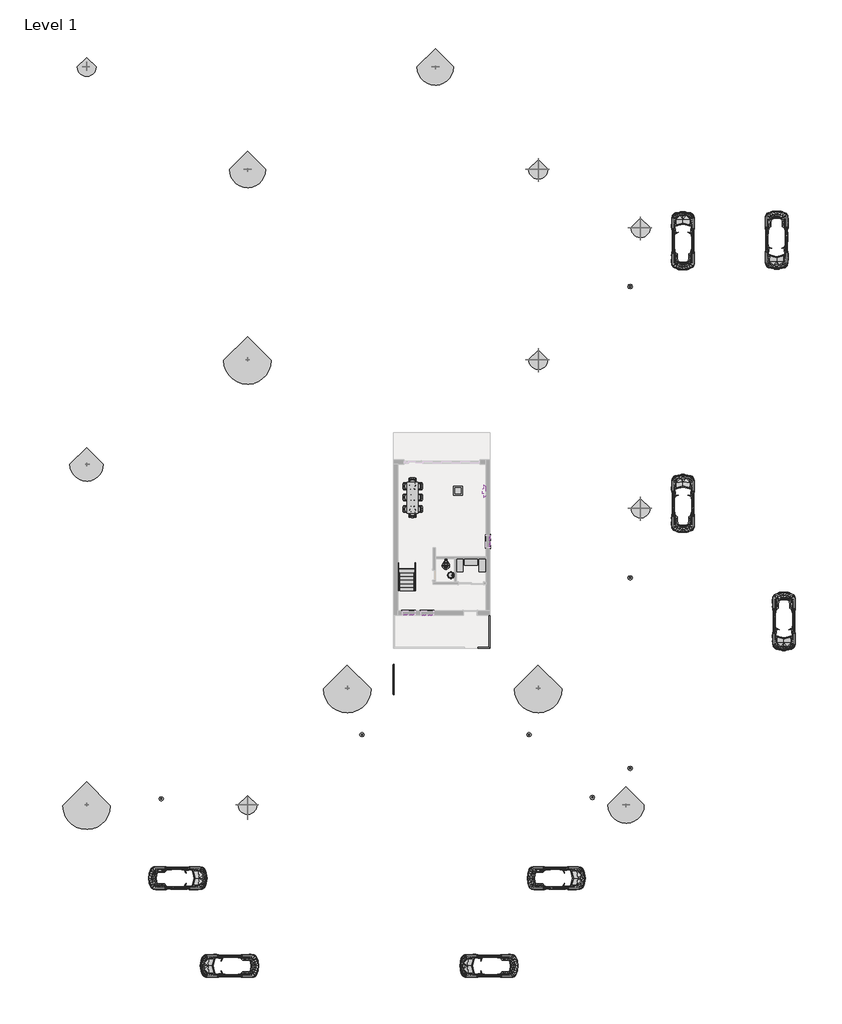
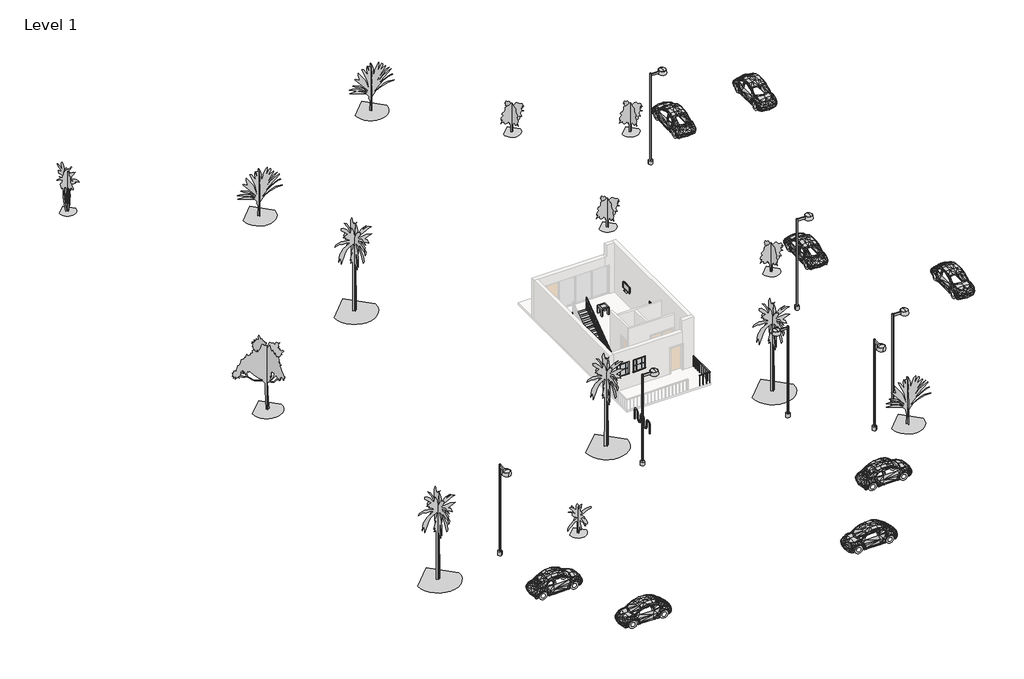
# One storey, part 2 of 2: 21 proxies, 14 furniture elements, 14 geographic elements, 7 light fixtures, 2 flow terminals, 2 members, 2 railings, 1 stair flight.
# Revit data of these elements (continued)
# Type "M_RPC Tree - Tropical" (continued)
#   built-in parameter 1005198 = "{2, 15},{39, RPC-16-G2M6-EAFX-C5H6-W000-ST1L-LVER-AU},{1, 0},{1, 0},{2, 35},{1, 8},{5, Color},{1, 0},{1, 0},{3, 0.8},{3, 0.8},{3, 0.8},{1, 8},{7, BBoxMin},{1, 0},{1, 0},{1, 0},{1, 0},{1, 0},{1, 8},{7, BBoxMax},{1, 0},{1, 0},{1, 0},{1, 0},{1, 0},{2, 11},{9, RPCTypeId},{1, 0},{1, 0},{39, RPC-16-G2M6-EAFX-C5H6-W000-ST1L-LVER-AU},{1, 6},{14, RPCPlantHeight},{1, 0},{1, 0},{7, 12.7953},{2, 11},{7, keyword},{1, 0},{1, 0},{74, :Geometry:RPC:Traveler's Palm:Ravenala madagascariensis:fan:palm:tropical.},{2, 11},{8, category},{1, 0},{1, 0},{17, :Trees [Tropical]},{2, 11},{12, LocalizedUID},{1, 0},{1, 0},{15, Traveler's Palm},{2, 14},{6, Height},{1, 0},{1, 0},{7, 12.7953},{1, 2},{16, Cast Reflections},{1, 0},{1, 0},{1, 0},{1, 2},{12, Cast Shadows},{1, 0},{1, 0},{1, 1},{1, 2},{9, Lock View},{1, 0},{1, 0},{1, 0},{1, 4},{5, ViewC},{1, 0},{1, 0},{1, 0},{2, 11},{20, AdvancedUIDefinition},{1, 0},{1, 0},{0, },{2, 11},{10, AssetLibID},{1, 0},{1, 0},{36, 4D3F6E72-3F99-4203-98E9-AF80B3C7A7A4},{2, 11},{10, BaseSchema},{1, 0},{1, 0},{9, RPCSchema},{2, 11},{12, ExchangeGUID},{1, 0},{1, 0},{0, },{1, 2},{6, Hidden},{1, 0},{1, 0},{1, 0},{1, 4},{11, RPCCategory},{1, 0},{1, 0},{1, 0},{2, 11},{8, RPCImage},{1, 0},{1, 0},{0, },{1, 4},{13, SchemaVersion},{1, 0},{1, 0},{1, 4},{2, 11},{12, UIDefinition},{1, 0},{1, 0},{0, },{2, 11},{6, UIName},{1, 0},{1, 0},{39, RPC-16-G2M6-EAFX-C5H6-W000-ST1L-LVER-AU},{2, 11},{11, VersionGUID},{1, 0},{1, 0},{9, RPCSchema},{2, 11},{9, assettype},{1, 0},{1, 0},{11, RPCGeometry},{2, 11},{11, description},{1, 0},{1, 0},{0, },{2, 11},{9, localname},{1, 0},{1, 0},{3, RPC},{2, 11},{9, localtype},{1, 0},{1, 0},{3, RPC},{1, 4},{8, revision},{1, 0},{1, 0},{1, 1},{2, 11},{9, thumbnail},{1, 0},{1, 0},{0, },{1, 4},{7, version},{1, 0},{1, 0},{1, 1},{1, 2},{20, RPC_Cast Reflections},{1, 0},{1, 0},{1, 1},{1, 2},{16, RPC_Cast Shadows},{1, 0},{1, 0},{1, 1},{1, 2},{13, RPC_Lock View},{1, 0},{1, 0},{1, 0},{1, 4},{9, RPC_ViewC},{1, 0},{1, 0},{1, 0},{21, assetlibrary_base.fbx},{1, 5},"
#   built-in parameter 1005195 = "RPC-16-G2M6-EAFX-C5H6-W000-ST1L-LVER-AU"
#   Height = 3900 mm
#   Plan Symbol = element 405753
#   Description = (empty or 0)
#   Default Elevation = 0
# Type "M_RPC Tree - Tropical"
#   built-in parameter 1005198 = "{2, 15},{39, RPC-16-G2MF-J1Q0-CAN1-N000-ST1L-LVER-AU},{1, 0},{1, 0},{2, 35},{1, 8},{5, Color},{1, 0},{1, 0},{3, 0.8},{3, 0.8},{3, 0.8},{1, 8},{7, BBoxMin},{1, 0},{1, 0},{1, 0},{1, 0},{1, 0},{1, 8},{7, BBoxMax},{1, 0},{1, 0},{1, 0},{1, 0},{1, 0},{2, 11},{9, RPCTypeId},{1, 0},{1, 0},{39, RPC-16-G2MF-J1Q0-CAN1-N000-ST1L-LVER-AU},{1, 6},{14, RPCPlantHeight},{1, 0},{1, 0},{7, 7.87402},{2, 11},{7, keyword},{1, 0},{1, 0},{75, :Geometry:RPC:Windmill Palm:Trachycarpus fortunei:in habitat:palm:tropical.},{2, 11},{8, category},{1, 0},{1, 0},{17, :Trees [Tropical]},{2, 11},{12, LocalizedUID},{1, 0},{1, 0},{13, Windmill Palm},{2, 14},{6, Height},{1, 0},{1, 0},{7, 7.87402},{1, 2},{16, Cast Reflections},{1, 0},{1, 0},{1, 0},{1, 2},{12, Cast Shadows},{1, 0},{1, 0},{1, 1},{1, 2},{9, Lock View},{1, 0},{1, 0},{1, 0},{1, 4},{5, ViewC},{1, 0},{1, 0},{1, 0},{2, 11},{20, AdvancedUIDefinition},{1, 0},{1, 0},{0, },{2, 11},{10, AssetLibID},{1, 0},{1, 0},{36, 4D3F6E72-3F99-4203-98E9-AF80B3C7A7A4},{2, 11},{10, BaseSchema},{1, 0},{1, 0},{9, RPCSchema},{2, 11},{12, ExchangeGUID},{1, 0},{1, 0},{0, },{1, 2},{6, Hidden},{1, 0},{1, 0},{1, 0},{1, 4},{11, RPCCategory},{1, 0},{1, 0},{1, 0},{2, 11},{8, RPCImage},{1, 0},{1, 0},{0, },{1, 4},{13, SchemaVersion},{1, 0},{1, 0},{1, 4},{2, 11},{12, UIDefinition},{1, 0},{1, 0},{0, },{2, 11},{6, UIName},{1, 0},{1, 0},{39, RPC-16-G2MF-J1Q0-CAN1-N000-ST1L-LVER-AU},{2, 11},{11, VersionGUID},{1, 0},{1, 0},{9, RPCSchema},{2, 11},{9, assettype},{1, 0},{1, 0},{11, RPCGeometry},{2, 11},{11, description},{1, 0},{1, 0},{0, },{2, 11},{9, localname},{1, 0},{1, 0},{3, RPC},{2, 11},{9, localtype},{1, 0},{1, 0},{3, RPC},{1, 4},{8, revision},{1, 0},{1, 0},{1, 1},{2, 11},{9, thumbnail},{1, 0},{1, 0},{0, },{1, 4},{7, version},{1, 0},{1, 0},{1, 1},{1, 2},{20, RPC_Cast Reflections},{1, 0},{1, 0},{1, 1},{1, 2},{16, RPC_Cast Shadows},{1, 0},{1, 0},{1, 1},{1, 2},{13, RPC_Lock View},{1, 0},{1, 0},{1, 0},{1, 4},{9, RPC_ViewC},{1, 0},{1, 0},{1, 0},{21, assetlibrary_base.fbx},{1, 5},"
#   built-in parameter 1005195 = "RPC-16-G2MF-J1Q0-CAN1-N000-ST1L-LVER-AU"
#   Height = 2400 mm
#   Plan Symbol = element 405753
#   Description = (empty or 0)
#   Default Elevation = 0
# Type "M_RPC Tree - Tropical : Cuban Royal Palm - 7.5 Meters"
#   built-in parameter 1005198 = "{2, 15},{39, RPC-16-FVGV-NKG0-7NHH-C000-ST1L-LVER-AU},{1, 0},{1, 0},{2, 35},{1, 8},{5, Color},{1, 0},{1, 0},{3, 0.8},{3, 0.8},{3, 0.8},{1, 8},{7, BBoxMin},{1, 0},{1, 0},{1, 0},{1, 0},{1, 0},{1, 8},{7, BBoxMax},{1, 0},{1, 0},{1, 0},{1, 0},{1, 0},{2, 11},{9, RPCTypeId},{1, 0},{1, 0},{39, RPC-16-FVGV-NKG0-7NHH-C000-ST1L-LVER-AU},{1, 6},{14, RPCPlantHeight},{1, 0},{1, 0},{7, 24.6063},{2, 11},{7, keyword},{1, 0},{1, 0},{72, :Geometry:RPC:Cuban Royal Palm:Roystonea regia (Oreodoxa):palm:tropical.},{2, 11},{8, category},{1, 0},{1, 0},{17, :Trees [Tropical]},{2, 11},{12, LocalizedUID},{1, 0},{1, 0},{16, Cuban Royal Palm},{2, 14},{6, Height},{1, 0},{1, 0},{7, 24.6063},{1, 2},{16, Cast Reflections},{1, 0},{1, 0},{1, 0},{1, 2},{12, Cast Shadows},{1, 0},{1, 0},{1, 1},{1, 2},{9, Lock View},{1, 0},{1, 0},{1, 0},{1, 4},{5, ViewC},{1, 0},{1, 0},{1, 0},{2, 11},{20, AdvancedUIDefinition},{1, 0},{1, 0},{0, },{2, 11},{10, AssetLibID},{1, 0},{1, 0},{36, 4D3F6E72-3F99-4203-98E9-AF80B3C7A7A4},{2, 11},{10, BaseSchema},{1, 0},{1, 0},{9, RPCSchema},{2, 11},{12, ExchangeGUID},{1, 0},{1, 0},{0, },{1, 2},{6, Hidden},{1, 0},{1, 0},{1, 0},{1, 4},{11, RPCCategory},{1, 0},{1, 0},{1, 0},{2, 11},{8, RPCImage},{1, 0},{1, 0},{0, },{1, 4},{13, SchemaVersion},{1, 0},{1, 0},{1, 4},{2, 11},{12, UIDefinition},{1, 0},{1, 0},{0, },{2, 11},{6, UIName},{1, 0},{1, 0},{39, RPC-16-FVGV-NKG0-7NHH-C000-ST1L-LVER-AU},{2, 11},{11, VersionGUID},{1, 0},{1, 0},{9, RPCSchema},{2, 11},{9, assettype},{1, 0},{1, 0},{11, RPCGeometry},{2, 11},{11, description},{1, 0},{1, 0},{0, },{2, 11},{9, localname},{1, 0},{1, 0},{3, RPC},{2, 11},{9, localtype},{1, 0},{1, 0},{3, RPC},{1, 4},{8, revision},{1, 0},{1, 0},{1, 1},{2, 11},{9, thumbnail},{1, 0},{1, 0},{0, },{1, 4},{7, version},{1, 0},{1, 0},{1, 1},{1, 2},{20, RPC_Cast Reflections},{1, 0},{1, 0},{1, 1},{1, 2},{16, RPC_Cast Shadows},{1, 0},{1, 0},{1, 1},{1, 2},{13, RPC_Lock View},{1, 0},{1, 0},{1, 0},{1, 4},{9, RPC_ViewC},{1, 0},{1, 0},{1, 0},{21, assetlibrary_base.fbx},{1, 5},"
#   built-in parameter 1005195 = "RPC-16-FVGV-NKG0-7NHH-C000-ST1L-LVER-AU"
#   Type Comments = "Cuban Royal Palm"
#   Height = 7500 mm
#   Plan Symbol = element 405753
#   Description = (empty or 0)
#   Default Elevation = 0
# Type "M_RPC Tree - Tropical : Grass Palm - 5.5 Meters"
#   built-in parameter 1005198 = "{2, 15},{39, RPC-16-FXGK-2WG0-PNFG-U000-ST1L-LVER-AU},{1, 0},{1, 0},{2, 35},{1, 8},{5, Color},{1, 0},{1, 0},{3, 0.8},{3, 0.8},{3, 0.8},{1, 8},{7, BBoxMin},{1, 0},{1, 0},{1, 0},{1, 0},{1, 0},{1, 8},{7, BBoxMax},{1, 0},{1, 0},{1, 0},{1, 0},{1, 0},{2, 11},{9, RPCTypeId},{1, 0},{1, 0},{39, RPC-16-FXGK-2WG0-PNFG-U000-ST1L-LVER-AU},{1, 6},{14, RPCPlantHeight},{1, 0},{1, 0},{7, 18.0446},{2, 11},{7, keyword},{1, 0},{1, 0},{76, :Geometry:RPC:Grass Palm:cordyline australis:grass palm:tropical:trees:beach},{2, 11},{8, category},{1, 0},{1, 0},{17, :Trees [Tropical]},{2, 11},{12, LocalizedUID},{1, 0},{1, 0},{10, Grass Palm},{2, 14},{6, Height},{1, 0},{1, 0},{7, 18.0446},{1, 2},{16, Cast Reflections},{1, 0},{1, 0},{1, 0},{1, 2},{12, Cast Shadows},{1, 0},{1, 0},{1, 1},{1, 2},{9, Lock View},{1, 0},{1, 0},{1, 0},{1, 4},{5, ViewC},{1, 0},{1, 0},{1, 0},{2, 11},{20, AdvancedUIDefinition},{1, 0},{1, 0},{0, },{2, 11},{10, AssetLibID},{1, 0},{1, 0},{36, 4D3F6E72-3F99-4203-98E9-AF80B3C7A7A4},{2, 11},{10, BaseSchema},{1, 0},{1, 0},{9, RPCSchema},{2, 11},{12, ExchangeGUID},{1, 0},{1, 0},{0, },{1, 2},{6, Hidden},{1, 0},{1, 0},{1, 0},{1, 4},{11, RPCCategory},{1, 0},{1, 0},{1, 0},{2, 11},{8, RPCImage},{1, 0},{1, 0},{0, },{1, 4},{13, SchemaVersion},{1, 0},{1, 0},{1, 4},{2, 11},{12, UIDefinition},{1, 0},{1, 0},{0, },{2, 11},{6, UIName},{1, 0},{1, 0},{39, RPC-16-FXGK-2WG0-PNFG-U000-ST1L-LVER-AU},{2, 11},{11, VersionGUID},{1, 0},{1, 0},{9, RPCSchema},{2, 11},{9, assettype},{1, 0},{1, 0},{11, RPCGeometry},{2, 11},{11, description},{1, 0},{1, 0},{0, },{2, 11},{9, localname},{1, 0},{1, 0},{3, RPC},{2, 11},{9, localtype},{1, 0},{1, 0},{3, RPC},{1, 4},{8, revision},{1, 0},{1, 0},{1, 1},{2, 11},{9, thumbnail},{1, 0},{1, 0},{0, },{1, 4},{7, version},{1, 0},{1, 0},{1, 1},{1, 2},{20, RPC_Cast Reflections},{1, 0},{1, 0},{1, 1},{1, 2},{16, RPC_Cast Shadows},{1, 0},{1, 0},{1, 1},{1, 2},{13, RPC_Lock View},{1, 0},{1, 0},{1, 0},{1, 4},{9, RPC_ViewC},{1, 0},{1, 0},{1, 0},{21, assetlibrary_base.fbx},{1, 5},"
#   built-in parameter 1005195 = "RPC-16-FXGK-2WG0-PNFG-U000-ST1L-LVER-AU"
#   Type Comments = "Grass Palm"
#   Height = 5500 mm
#   Plan Symbol = element 405753
#   Description = (empty or 0)
#   Default Elevation = 0
# Type "M_RPC Tree - Tropical : Hurricane Palm - 3.6 Meters"
#   built-in parameter 1005198 = "{2, 15},{39, RPC-16-FXGL-UL7X-PH44-0000-ST1L-LVER-AU},{1, 0},{1, 0},{2, 35},{1, 8},{5, Color},{1, 0},{1, 0},{3, 0.8},{3, 0.8},{3, 0.8},{1, 8},{7, BBoxMin},{1, 0},{1, 0},{1, 0},{1, 0},{1, 0},{1, 8},{7, BBoxMax},{1, 0},{1, 0},{1, 0},{1, 0},{1, 0},{2, 11},{9, RPCTypeId},{1, 0},{1, 0},{39, RPC-16-FXGL-UL7X-PH44-0000-ST1L-LVER-AU},{1, 6},{14, RPCPlantHeight},{1, 0},{1, 0},{6, 11.811},{2, 11},{7, keyword},{1, 0},{1, 0},{102, :Geometry:RPC:Hurricane Palm:Ptychosperma macarthurii (New Guinea):with jagged leaftips:palm:tropical.},{2, 11},{8, category},{1, 0},{1, 0},{17, :Trees [Tropical]},{2, 11},{12, LocalizedUID},{1, 0},{1, 0},{14, Hurricane Palm},{2, 14},{6, Height},{1, 0},{1, 0},{6, 11.811},{1, 2},{16, Cast Reflections},{1, 0},{1, 0},{1, 0},{1, 2},{12, Cast Shadows},{1, 0},{1, 0},{1, 1},{1, 2},{9, Lock View},{1, 0},{1, 0},{1, 0},{1, 4},{5, ViewC},{1, 0},{1, 0},{1, 0},{2, 11},{20, AdvancedUIDefinition},{1, 0},{1, 0},{0, },{2, 11},{10, AssetLibID},{1, 0},{1, 0},{36, 4D3F6E72-3F99-4203-98E9-AF80B3C7A7A4},{2, 11},{10, BaseSchema},{1, 0},{1, 0},{9, RPCSchema},{2, 11},{12, ExchangeGUID},{1, 0},{1, 0},{0, },{1, 2},{6, Hidden},{1, 0},{1, 0},{1, 0},{1, 4},{11, RPCCategory},{1, 0},{1, 0},{1, 0},{2, 11},{8, RPCImage},{1, 0},{1, 0},{0, },{1, 4},{13, SchemaVersion},{1, 0},{1, 0},{1, 4},{2, 11},{12, UIDefinition},{1, 0},{1, 0},{0, },{2, 11},{6, UIName},{1, 0},{1, 0},{39, RPC-16-FXGL-UL7X-PH44-0000-ST1L-LVER-AU},{2, 11},{11, VersionGUID},{1, 0},{1, 0},{9, RPCSchema},{2, 11},{9, assettype},{1, 0},{1, 0},{11, RPCGeometry},{2, 11},{11, description},{1, 0},{1, 0},{0, },{2, 11},{9, localname},{1, 0},{1, 0},{3, RPC},{2, 11},{9, localtype},{1, 0},{1, 0},{3, RPC},{1, 4},{8, revision},{1, 0},{1, 0},{1, 1},{2, 11},{9, thumbnail},{1, 0},{1, 0},{0, },{1, 4},{7, version},{1, 0},{1, 0},{1, 1},{1, 2},{20, RPC_Cast Reflections},{1, 0},{1, 0},{1, 1},{1, 2},{16, RPC_Cast Shadows},{1, 0},{1, 0},{1, 1},{1, 2},{13, RPC_Lock View},{1, 0},{1, 0},{1, 0},{1, 4},{9, RPC_ViewC},{1, 0},{1, 0},{1, 0},{21, assetlibrary_base.fbx},{1, 5},"
#   built-in parameter 1005195 = "RPC-16-FXGL-UL7X-PH44-0000-ST1L-LVER-AU"
#   Type Comments = "Hurricane Palm"
#   Height = 3600 mm
#   Plan Symbol = element 405753
#   Description = (empty or 0)
#   Default Elevation = 0
# Type "M_RPC Tree - Tropical : Japanese Fiber Banana - 2.4 Meters"
#   built-in parameter 1005198 = "{2, 15},{39, RPC-16-FVGT-NR7X-7G1M-A000-ST1L-LVER-AU},{1, 0},{1, 0},{2, 35},{1, 8},{5, Color},{1, 0},{1, 0},{3, 0.8},{3, 0.8},{3, 0.8},{1, 8},{7, BBoxMin},{1, 0},{1, 0},{1, 0},{1, 0},{1, 0},{1, 8},{7, BBoxMax},{1, 0},{1, 0},{1, 0},{1, 0},{1, 0},{2, 11},{9, RPCTypeId},{1, 0},{1, 0},{39, RPC-16-FVGT-NR7X-7G1M-A000-ST1L-LVER-AU},{1, 6},{14, RPCPlantHeight},{1, 0},{1, 0},{7, 7.87402},{2, 11},{7, keyword},{1, 0},{1, 0},{62, :Geometry:RPC:Japanese Fiber Banana:Musa basjoo:Tree:Tropical.},{2, 11},{8, category},{1, 0},{1, 0},{17, :Trees [Tropical]},{2, 11},{12, LocalizedUID},{1, 0},{1, 0},{21, Japanese Fiber Banana},{2, 14},{6, Height},{1, 0},{1, 0},{7, 7.87402},{1, 2},{16, Cast Reflections},{1, 0},{1, 0},{1, 0},{1, 2},{12, Cast Shadows},{1, 0},{1, 0},{1, 1},{1, 2},{9, Lock View},{1, 0},{1, 0},{1, 0},{1, 4},{5, ViewC},{1, 0},{1, 0},{1, 0},{2, 11},{20, AdvancedUIDefinition},{1, 0},{1, 0},{0, },{2, 11},{10, AssetLibID},{1, 0},{1, 0},{36, 4D3F6E72-3F99-4203-98E9-AF80B3C7A7A4},{2, 11},{10, BaseSchema},{1, 0},{1, 0},{9, RPCSchema},{2, 11},{12, ExchangeGUID},{1, 0},{1, 0},{0, },{1, 2},{6, Hidden},{1, 0},{1, 0},{1, 0},{1, 4},{11, RPCCategory},{1, 0},{1, 0},{1, 0},{2, 11},{8, RPCImage},{1, 0},{1, 0},{0, },{1, 4},{13, SchemaVersion},{1, 0},{1, 0},{1, 4},{2, 11},{12, UIDefinition},{1, 0},{1, 0},{0, },{2, 11},{6, UIName},{1, 0},{1, 0},{39, RPC-16-FVGT-NR7X-7G1M-A000-ST1L-LVER-AU},{2, 11},{11, VersionGUID},{1, 0},{1, 0},{9, RPCSchema},{2, 11},{9, assettype},{1, 0},{1, 0},{11, RPCGeometry},{2, 11},{11, description},{1, 0},{1, 0},{0, },{2, 11},{9, localname},{1, 0},{1, 0},{3, RPC},{2, 11},{9, localtype},{1, 0},{1, 0},{3, RPC},{1, 4},{8, revision},{1, 0},{1, 0},{1, 1},{2, 11},{9, thumbnail},{1, 0},{1, 0},{0, },{1, 4},{7, version},{1, 0},{1, 0},{1, 1},{1, 2},{20, RPC_Cast Reflections},{1, 0},{1, 0},{1, 1},{1, 2},{16, RPC_Cast Shadows},{1, 0},{1, 0},{1, 1},{1, 2},{13, RPC_Lock View},{1, 0},{1, 0},{1, 0},{1, 4},{9, RPC_ViewC},{1, 0},{1, 0},{1, 0},{21, assetlibrary_base.fbx},{1, 5},"
#   built-in parameter 1005195 = "RPC-16-FVGT-NR7X-7G1M-A000-ST1L-LVER-AU"
#   Type Comments = "Japanese Fiber Banana"
#   Height = 2400 mm
#   Plan Symbol = element 405753
#   Description = (empty or 0)
#   Default Elevation = 0
# Type "M_Street Light - Standard"
#   Photometric Web File = "SLS1ET18.ies"
#   Lamp = "E-18"
#   Wattage Comments = "250"
#   Wattage = 250 W
#   built-in parameter 1150110 = 1 (stored number, unit not read)
#   built-in parameter 1114217 = 1 (stored number, unit not read)
#   built-in parameter 1150109 = 1 (stored number, unit not read)
#   built-in parameter 1150113 = 1 (stored number, unit not read)
#   Tilt Angle = 90.00°
#   built-in parameter 1150115 = 1 (stored number, unit not read)
#   built-in parameter 1150105 = 2307.75 (stored number, unit not read)
#   built-in parameter 1150112 = 1 (stored number, unit not read)
#   built-in parameter 1150114 = 1 (stored number, unit not read)
#   built-in parameter 1150107 = 4000 (stored number, unit not read)
#   built-in parameter 1150106 = 23.0775 (stored number, unit not read)
#   Height = 7500 mm
#   Lumens = 29000 lm
#   built-in parameter 1150104 = 10.7768 (stored number, unit not read)
#   Voltage = 480 V
#   built-in parameter 1114218 = 1 (stored number, unit not read)
#   built-in parameter 1150133 = 10 (stored number, unit not read)
#   Apparent Load = 250 VA
#   built-in parameter 1150134 = 12
#   built-in parameter 1150137 = 1
#   Color Filter = 16777215
#   Number of poles = 3
#   Stand Material = Steel, Paint Finish, Dark Gray, Matte
#   Shade Material = Steel, Paint Finish, Dark Gray, Matte
#   Load Classification = Lighting - Exterior
#   Diffuser Material = Glass, Frosted
#   Dimming Lamp Color Temperature Shift = (empty or 0)
#   Default Elevation = 0
# Type "M_Street Light - Standard : 250W Halogen - 277V"
#   Photometric Web File = "SLS1T4.IES"
#   Lamp = "T-4"
#   Wattage Comments = "250"
#   Wattage = 250 W
#   built-in parameter 1150110 = 1 (stored number, unit not read)
#   built-in parameter 1114217 = 1 (stored number, unit not read)
#   built-in parameter 1150109 = 1 (stored number, unit not read)
#   built-in parameter 1150113 = 1 (stored number, unit not read)
#   Tilt Angle = -90.00°
#   built-in parameter 1150115 = 1 (stored number, unit not read)
#   built-in parameter 1150105 = 397.887 (stored number, unit not read)
#   built-in parameter 1150112 = 1 (stored number, unit not read)
#   built-in parameter 1150114 = 1 (stored number, unit not read)
#   built-in parameter 1150107 = 3200 (stored number, unit not read)
#   built-in parameter 1150106 = 3.97887 (stored number, unit not read)
#   Height = 7500 mm
#   Lumens = 5000 lm
#   built-in parameter 1150104 = 1.85806 (stored number, unit not read)
#   Voltage = 277 V
#   built-in parameter 1114218 = 1 (stored number, unit not read)
#   built-in parameter 1150133 = 10 (stored number, unit not read)
#   Apparent Load = 250 VA
#   built-in parameter 1150134 = 3
#   built-in parameter 1150137 = 1
#   Color Filter = 16777215
#   Number of poles = 1
#   Stand Material = Steel, Paint Finish, Dark Gray, Matte
#   Shade Material = Steel, Paint Finish, Dark Gray, Matte
#   Load Classification = Lighting - Exterior
#   Diffuser Material = Glass, Frosted
#   Dimming Lamp Color Temperature Shift = (empty or 0)
#   Default Elevation = 0
# Type "M_Street Light - Standard : 400W Halogen - 120V"
#   Photometric Web File = "SLS1T3.ies"
#   Lamp = "T-3"
#   Wattage Comments = "400"
#   Wattage = 400 W
#   built-in parameter 1150110 = 1 (stored number, unit not read)
#   built-in parameter 1114217 = 1 (stored number, unit not read)
#   built-in parameter 1150109 = 1 (stored number, unit not read)
#   built-in parameter 1150113 = 1 (stored number, unit not read)
#   Tilt Angle = -90.00°
#   built-in parameter 1150115 = 1 (stored number, unit not read)
#   built-in parameter 1150105 = 795.775 (stored number, unit not read)
#   built-in parameter 1150112 = 1 (stored number, unit not read)
#   built-in parameter 1150114 = 1 (stored number, unit not read)
#   built-in parameter 1150107 = 3200 (stored number, unit not read)
#   built-in parameter 1150106 = 7.95775 (stored number, unit not read)
#   Height = 7500 mm
#   Lumens = 10000 lm
#   built-in parameter 1150104 = 2.32258 (stored number, unit not read)
#   Voltage = 120 V
#   built-in parameter 1114218 = 1 (stored number, unit not read)
#   built-in parameter 1150133 = 10 (stored number, unit not read)
#   Apparent Load = 400 VA
#   built-in parameter 1150134 = 3
#   built-in parameter 1150137 = 1
#   Color Filter = 16777215
#   Number of poles = 1
#   Stand Material = Steel, Paint Finish, Dark Gray, Matte
#   Shade Material = Steel, Paint Finish, Dark Gray, Matte
#   Load Classification = Lighting - Exterior
#   Diffuser Material = Glass, Frosted
#   Dimming Lamp Color Temperature Shift = (empty or 0)
#   Default Elevation = 0
# Type "900mm Pipe"
#   built-in parameter 1008612 = 0.019685 (stored number, unit not read)
#   built-in parameter 1008611 = 0.0984252 (stored number, unit not read)
#   built-in parameter 1008609 = 3.28084 (stored number, unit not read)
#   built-in parameter 1008604 = 0.19685 (stored number, unit not read)
#   built-in parameter 1008603 = 0.164042 (stored number, unit not read)
#   Railing Height = 900 mm
#   built-in parameter 1008630 = 2
#   built-in parameter 1008610 = 1
#   built-in parameter 1008605 = 1
#   built-in parameter 1008618 = M_Baluster - Round : 25mm
# Type "NEW RAILING"
#   built-in parameter 1008612 = 0.019685 (stored number, unit not read)
#   built-in parameter 1008611 = 0.019685 (stored number, unit not read)
#   built-in parameter 1008609 = 0.902231 (stored number, unit not read)
#   built-in parameter 1008604 = 0.19685 (stored number, unit not read)
#   built-in parameter 1008603 = 0.164042 (stored number, unit not read)
#   Railing Height = 900 mm
#   built-in parameter 1008630 = 2
#   built-in parameter 1008610 = 2
#   built-in parameter 1008608 = 1
#   built-in parameter 1008618 = M_Baluster - Square : 20mm
# Element 1 (IfcBuildingElementProxy, "M_Bicycle Rack : M_Bicycle Rack")
#   Phase Created = New Construction
# Elements 2, 3, 4, 5, 6, 7 (IfcBuildingElementProxy, "M_Muntin Pattern_2x2 : M_Muntin Pattern_2x2")
#   Width = 288.475 mm
#   Height = 760.3 mm
#   Interior Material = Wood - Stained
#   Exterior Material = Clad - White
#   Phase Created = New Construction
#   Materials on its faces: "Clad - White", "Wood - Stained"
# Elements 8, 9, 10, 11, 12, 13, 14, 15 (IfcBuildingElementProxy, "M_RPC Beetle : M_RPC Beetle")
#   Phase Created = New Construction
# Elements 16, 17, 18 (IfcBuildingElementProxy, "M_Trim-Window-Exterior-Flat : with Sill")
#   Opening Width = 850 mm
#   Opening Height = 900 mm
#   Trim Material = Clad - White
#   Phase Created = New Construction
#   Materials on its faces: "Clad - White"
# Elements 19, 20, 21 (IfcBuildingElementProxy, "M_Trim-Window-Interior-Flat : Picture Frame")
#   Opening Width = 850 mm
#   Opening Height = 900 mm
#   Trim Material = Wood - Stained
#   Phase Created = New Construction
#   Materials on its faces: "Wood - Stained"
# Element 22 (IfcFlowTerminal, "M_Sink Vanity-Round : 482 x 482mm")
#   Top Of Counter = 750 mm
#   Phase Created = New Construction
#   Materials on its faces: "Porcelain, Linen", "Steel, Polished"
# Element 23 (IfcFlowTerminal, "M_Toilet-Commercial-Wall-3D : 380mm Seat Height")
#   Phase Created = New Construction
#   Materials on its faces: "Laminate, Ivory, Matte", "Porcelain, Ivory", "Steel, Polished"
# Element 24 (IfcFurniture, "0810mm")
#   Stand = yes
#   Phase Created = New Construction
#   Materials on its faces: "TV - Black", "TV - Glass", "TV - Screen"
# Elements 25, 26, 27 (IfcFurniture, "M_Furniture_System-Storage-Cabinet-2_Vertical_File : 900 x 450 x 650mm")
#   Show Solid = yes
#   Show Dashed = no
#   Drawer Finish = Metal - Paint - Beige
#   Cabinet Material = Metal - Paint - Beige
#   Phase Created = New Construction
#   Materials on its faces: "Metal - Paint - Beige"
# Elements 28, 29, 30, 31, 32, 33, 34, 35 (IfcFurniture, "M_Seating-Auditorium : 457 x 610mm")
#   Phase Created = New Construction
#   Materials on its faces: "Steel, Paint Finish, Dark Gray, Matte", "Linen, Beige"
# Element 36 (IfcFurniture, "M_Table-Coffee : 0610 x 0610 x 0610mm")
#   Phase Created = New Construction
#   Materials on its faces: "Wood - Teak", "Steel, Chrome Plated", "Glass - Clear, Grey"
# Element 37 (IfcFurniture, "M_Table-Dining : 0762 x 2134mm")
#   Phase Created = New Construction
#   Materials on its faces: "Steel, Chrome Plated", "Glass - Clear, Grey"
# Elements 38, 39, 40, 41, 42, 43, 44 (IfcGeographicElement, "M_RPC Tree - Tropical")
#   Phase Created = New Construction
# Elements 45, 46, 47, 48 (IfcGeographicElement, "M_RPC Tree - Tropical : Cuban Royal Palm - 7.5 Meters")
#   Phase Created = New Construction
# Element 49 (IfcGeographicElement, "M_RPC Tree - Tropical : Grass Palm - 5.5 Meters")
#   Phase Created = New Construction
# Element 50 (IfcGeographicElement, "M_RPC Tree - Tropical : Hurricane Palm - 3.6 Meters")
#   Phase Created = New Construction
# Element 51 (IfcGeographicElement, "M_RPC Tree - Tropical : Japanese Fiber Banana - 2.4 Meters")
#   Phase Created = New Construction
# Element 52 (IfcLightFixture, "M_Street Light - Standard")
#   Phase Created = New Construction
#   Materials on its faces: "Steel, Paint Finish, Dark Gray, Matte", "Glass, Frosted"
# Element 53 (IfcLightFixture, "M_Street Light - Standard : 250W Halogen - 277V")
#   Phase Created = New Construction
#   Materials on its faces: "Steel, Paint Finish, Dark Gray, Matte", "Glass, Frosted"
# Elements 54, 55, 56, 57, 58 (IfcLightFixture, "M_Street Light - Standard : 400W Halogen - 120V")
#   Phase Created = New Construction
#   Materials on its faces: "Steel, Paint Finish, Dark Gray, Matte", "Glass, Frosted"
# Elements 59, 60 (IfcMember, "Stringer - 50mm Width")
#   Phase Created = New Construction
# Element 61 (IfcRailing, "900mm Pipe")
#   Phase Created = New Construction
# Element 62 (IfcRailing, "NEW RAILING")
#   Phase Created = New Construction
#   Materials on its faces: "Default New Material"
# Element 63 (IfcStairFlight, "50mm Tread 13mm Riser")
#   Phase Created = New Construction
# Materials
#   "Porcelain, Linen": class "Ceramic", colour RGB 249 239 230, transparency 0, Description = "Porcelain, linen", Cost = 0
#   "Steel, Polished": class "Metal", colour RGB 57 57 57, transparency 0, Description = "Polished steel", Cost = 0
#   "Porcelain, Ivory": class "Ceramic", colour RGB 247 247 239, transparency 0, Description = "Porcelain, ivory", Cost = 0
#   "Laminate, Ivory, Matte": class "Plastic", colour RGB 247 247 239, transparency 0, Description = "Plastic Laminate - Ivory, Matte", Cost = 0
#   "Metal - Paint - Beige": class "Metal", colour RGB 247 225 182, transparency 0
#   "Linen, Beige": class "Textile", colour RGB 249 239 230, transparency 0, Description = "Linen, beige", Cost = 0
#   "Steel, Paint Finish, Dark Gray, Matte": class "Metal", colour RGB 0 0 0, transparency 0, Description = "Steel, paint finish, dark gray, matte", Cost = 0
#   "Steel, Chrome Plated": class "Metal", colour RGB 17 17 17, transparency 0, Description = "Chromiuim plated steel", Cost = 0
#   "Wood - Teak": class "Wood", colour RGB 145 112 90, transparency 0
#   "Glass - Clear, Grey": class "Glass", colour RGB 252 255 255, transparency 0.64
#   "Glass, Frosted": class "Glass", colour RGB 249 250 249, transparency 0.8, Description = "physical material", Cost = 0
#   "Clad - White": class "Wood", colour RGB 242 242 238, transparency 0, Cost = 0
#   "Wood - Stained": class "Wood", colour RGB 224 178 126, transparency 0, Cost = 0
#   "TV - Black": colour RGB 49 49 49, transparency 0
#   "TV - Glass": colour RGB 157 157 157, transparency 0.9
#   "TV - Screen": colour RGB 0 0 0, transparency 0
#   "Default New Material": class "Generic", colour RGB 211 206 0, transparency 0.8, Cost = 0
